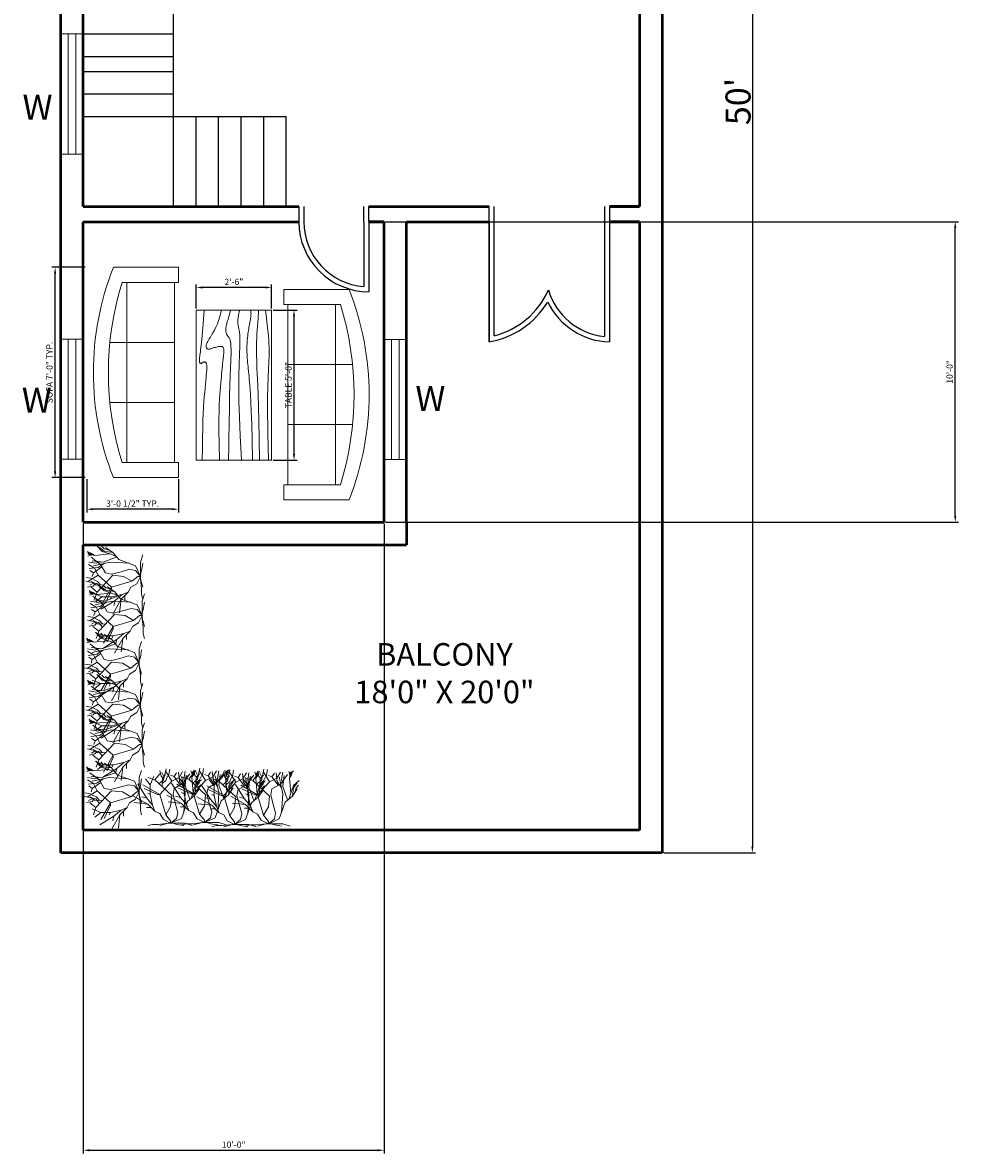
# Model space of a CAD drawing. Units: inches. Extents: x 995 to 2141, y 2161 to 2928.
# Tile 6 of 7: x 1768 to 2141, y 2161 to 2613. Entities that reach past the tile are written whole.
import ezdxf

# ---------------------------------------------------------------- set-up
doc = ezdxf.new("R2010")
doc.units = ezdxf.units.IN
for name, color, linetype, lineweight in [('A-ANNO-DIMS', 2, 'Continuous', 18), ('A-ANNO-TEXT', 7, 'Continuous', 18), ('A-AREA-IDEN', 7, 'Continuous', 25), ('A-DOOR', 3, 'Continuous', 25), ('A-FLOR-STRS', 7, 'Continuous', 25), ('A-FURN', 8, 'Continuous', 18), ('A-GLAZ', 4, 'Continuous', 18), ('A-WALL', 7, 'Continuous', 50), ('L-PLNT-TREE', 94, 'Continuous', 13)]:
    doc.layers.add(name, color=color, linetype=linetype, lineweight=lineweight)
doc.styles.get("Standard").update_dxf_attribs({"font": 'arial.ttf'})
doc.dimstyles.new('ISO-25', dxfattribs={"dimtxt": 2.5, "dimasz": 2.5, "dimexe": 1.25, "dimexo": 0.625, "dimtad": 1, "dimdec": 0, "dimlunit": 3, "dimtxsty": 'Standard', "dimcen": 2.5, "dimadec": 0, "dimazin": 0, "dimtfac": 1, "dimtdec": 0, "dimtmove": 0, "dimatfit": 3, "dimfxl": 1, "dimarcsym": 0})

# ---------------------------------------------------------------- blocks, each defined once
blk = doc.blocks.new('*U15')
for p, q in [((-11.433, 18.289), (-10.457, 22.749)), ((-9.48, 19.775), (-8.992, 22.592)), ((-16.8, 16.32), (-18.72, 18.72)), ((-14.88, 18.24), (-17.76, 19.2)), ((-16.8, 16.32), (-15.36, 19.68)), ((-14.88, 18.24), (-12.96, 20.64)), ((-8.16, 12), (-14.88, 18.24)), ((-13.325, 16.724), (-11.433, 18.289)), ((-12.471, 19.775), (-12.898, 22.044)), ((-11.677, 19.071), (-12.471, 19.775)), ((-11.28, 19.619), (-12.104, 21.184)), ((-12.043, 15.628), (-11.921, 18.836)), ((-11.921, 18.836), (-10.64, 20.401)), ((-10.579, 18.054), (-9.846, 19.697)), ((-8.16, 17.76), (-10.56, 21.6)), ((-7.2, 19.68), (-8.64, 20.16)), ((-8.16, 17.76), (-5.28, 19.2)), ((-7.2, 19.68), (-6.24, 21.12)), ((-4.8, 16.32), (-7.2, 19.68)), ((-5.086, 17.741), (-5.513, 21.34)), ((-5.28, 19.2), (-3.84, 21.6)), ((-2.88, 12.96), (-4.32, 19.68)), ((-3.84, 16.8), (-0.96, 20.64)), ((-3.377, 18.602), (-2.888, 21.575)), ((-2.766, 16.802), (-3.377, 18.602)), ((-2.88, 15.84), (-2.4, 20.16)), ((-0.508, 21.888), (-0.081, 20.558)), ((-0.203, 19.149), (0.102, 21.34)), ((0.346, 13.203), (-0.203, 19.149)), ((-0.142, 19.384), (0.59, 20.401)), ((-0.02, 20.01), (0.896, 21.105)), ((0.041, 20.714), (1.384, 22.044)), ((0.102, 21.34), (0.835, 21.888)), ((1.323, 16.254), (3.642, 18.289)), ((-18.24, 11.04), (-21.755, 16.655)), ((-12.96, 12.48), (-19.68, 16.32)), ((-13.92, 12.48), (-19.2, 14.88)), ((-16.8, 12.48), (-16.8, 16.32)), ((-12.96, 12.48), (-8.16, 17.76)), ((-11.982, 16.802), (-10.579, 18.054)), ((-7.68, 12.48), (-7.2, 14.88)), ((-7.2, 14.88), (-3.84, 16.8)), ((-3.377, 15.315), (-5.086, 17.819)), ((-0.96, 10.56), (-2.88, 15.84)), ((0.346, 13.203), (1.323, 16.254)), ((0.96, 12), (1.44, 15.36)), ((0.96, 12), (2.88, 14.88)), ((1.44, 15.36), (2.88, 17.28)), ((1.92, 13.44), (2.4, 15.36)), ((2.4, 15.36), (3.36, 16.32)), ((-17.76, 8.64), (-23.663, 11.961)), ((-17.76, 8.64), (-23.128, 9.222)), ((-18.24, 11.04), (-20.16, 11.52)), ((-15.84, 8.16), (-18.24, 11.04)), ((-16.8, 12.48), (-17.76, 12.96)), ((-15.84, 8.16), (-16.8, 12.48)), ((-12.96, 12.48), (-13.92, 12.48)), ((-10.56, 4.32), (-12.96, 12.48)), ((-8.64, 7.68), (-8.16, 12)), ((-6.72, 8.64), (-7.68, 12.48)), ((-4.32, 2.88), (-1.92, 9.6)), ((-3.36, 5.28), (-2.88, 12.96)), ((-1.92, 9.6), (0.96, 12)), ((-0.48, 10.8), (0.346, 13.203)), ((-16.32, 7.2), (-18.24, 7.2)), ((-14.88, 5.76), (-17.76, 8.64)), ((-14.88, 5.76), (-15.84, 8.16)), ((-12.96, 4.8), (-14.88, 5.76)), ((-11.52, 2.4), (-12.96, 4.8)), ((-10.56, 4.32), (-8.64, 7.68)), ((-5.76, 5.28), (-6.72, 8.64)), ((-6.24, 2.88), (-5.76, 5.28)), ((-15.84, 0.48), (-17.76, 0)), ((-13.44, 0.48), (-15.84, 0.48)), ((-9.6, 0.96), (-13.44, 0.48)), ((-9.6, 0.96), (-12.96, 0)), ((-8.64, 0.96), (-11.52, 2.4)), ((-8.64, 1.92), (-10.56, 4.32)), ((-9.6, 0.96), (-7.68, 0.96)), ((-8.64, 0.96), (-4.32, 2.88)), ((-8.64, 0.96), (-6.24, 2.88)), ((-8.64, 0.96), (-8.64, 1.92)), ((-8.64, 0.96), (-2.88, 0.96)), ((-7.68, 0.96), (-6.24, 0.48)), ((-6.24, 0.48), (-3.36, 0)), ((-2.88, 0.96), (0, 0))]:
    blk.add_line(p, q)
blk = doc.blocks.new('Sofa - Roundback 7 ft.')
for p, q in [((-12.00002, -32.4421), (-12.00003, -6.5971)), ((11.99997, -32.4421), (11.99998, -6.5971)), ((-36.000027, -34), (-36.000027, -11.4696)), ((-35.999844, -13.3819), (35.9998, -13.3819)), ((35.99998, -34), (35.99998, -11.4696)), ((-36.000027, -32.4421), (35.99998, -32.4421))]:
    blk.add_line(p, q)
for points in [[(-36.000027, -34), (-42.000027, -34), (-42.000027, -8)], [(41.99998, -8), (41.99998, -34), (35.99998, -34)]]:
    blk.add_lwpolyline(points)
for centre, radius, start, end in [((0, -114.25), 114.25, 68.43141, 111.5686), ((-0.00001, -127.1968), 121.1968, 72.72033, 107.2797)]:
    blk.add_arc(centre, radius, start, end)
blk = doc.blocks.new('Table - Rectangular Woodgrain 60 x 30 in.')
for p, q in [((0, 0), (0, -30)), ((60, 0), (0, 0)), ((60, -30), (60, 0)), ((0, -30), (60, -30))]:
    blk.add_line(p, q)
for points in [[(0, -2.4), (4.8155, -2.418), (9.0302, -2.4688), (12.709, -2.5477), (15.9167, -2.65), (18.7181, -2.7711), (21.1781, -2.9063), (23.3616, -3.0508), (25.3333, -3.2), (27.1477, -3.3495), (28.8172, -3.4958), (30.3437, -3.636), (31.7291, -3.7667), (32.9756, -3.8849), (34.0849, -3.9875), (35.059, -4.0714), (35.9, -4.1334), (36.6114, -4.1711), (37.2041, -4.1854), (37.6906, -4.1779), (38.0833, -4.15), (38.3948, -4.1034), (38.6375, -4.0396), (38.8239, -3.9602), (38.9666, -3.8667), (39.0764, -3.7608), (39.1573, -3.6448), (39.2116, -3.521), (39.2416, -3.3917), (39.2498, -3.2593), (39.2385, -3.1261), (39.21, -2.9944), (39.1666, -2.8667), (39.111, -2.7447), (39.0468, -2.6281), (38.978, -2.5163), (38.9083, -2.4083), (38.8418, -2.3035), (38.7823, -2.201), (38.7337, -2.1001), (38.7, -2), (38.6844, -1.9003), (38.6875, -1.8021), (38.7094, -1.707), (38.75, -1.6167), (38.8094, -1.5326), (38.8875, -1.4563), (38.9844, -1.3893), (39.1, -1.3333), (39.2351, -1.2896), (39.3937, -1.2583), (39.5804, -1.2396), (39.8, -1.2333), (40.057, -1.2396), (40.3562, -1.2583), (40.7023, -1.2896), (41.1, -1.3333), (41.5547, -1.3895), (42.0755, -1.4573), (42.6721, -1.5361), (43.3542, -1.625), (44.1316, -1.7233), (45.014, -1.8302), (46.0114, -1.9449), (47.1333, -2.0667), (48.3862, -2.1947), (49.7625, -2.3281), (51.2513, -2.4663), (52.8416, -2.6083), (54.5226, -2.7535), (56.2833, -2.9011), (58.1127, -3.0501), (60, -3.2)], [(0, -9.2), (6.5759, -9.0858), (11.9385, -9.0365), (16.2527, -9.0418), (19.6833, -9.0917), (22.3952, -9.1759), (24.5531, -9.2844), (26.322, -9.4069), (27.8666, -9.5333), (29.3241, -9.6553), (30.7203, -9.7719), (32.0532, -9.8837), (33.3208, -9.9917), (34.5213, -10.0965), (35.6526, -10.199), (36.7128, -10.2999), (37.7, -10.4), (38.6129, -10.4996), (39.4531, -10.5969), (40.223, -10.6895), (40.925, -10.775), (41.5613, -10.8512), (42.1344, -10.9156), (42.6465, -10.966), (43.1, -11), (43.4976, -11.0158), (43.8437, -11.0136), (44.143, -10.9942), (44.4, -10.9583), (44.6195, -10.9069), (44.8062, -10.8406), (44.9648, -10.7603), (45.1, -10.6667), (45.2155, -10.5598), (45.3114, -10.4365), (45.3871, -10.2929), (45.4416, -10.125), (45.4743, -9.929), (45.4844, -9.7011), (45.4709, -9.4371), (45.4333, -9.1333), (45.3716, -8.7883), (45.2896, -8.4104), (45.1919, -8.0107), (45.0833, -7.6), (44.9685, -7.1893), (44.8521, -6.7896), (44.7388, -6.4117), (44.6333, -6.0667), (44.54, -5.7628), (44.4614, -5.4979), (44.4001, -5.2675), (44.3583, -5.0667), (44.3384, -4.8909), (44.3427, -4.7354), (44.3736, -4.5956), (44.4333, -4.4667), (44.5236, -4.3453), (44.6427, -4.2333), (44.7884, -4.1339), (44.9583, -4.05), (45.1501, -3.9849), (45.3614, -3.9417), (45.59, -3.9234), (45.8333, -3.9333), (46.0915, -3.9749), (46.3734, -4.0531), (46.6906, -4.1736), (47.0542, -4.3417), (47.4756, -4.5629), (47.9661, -4.8427), (48.5372, -5.1866), (49.2, -5.6), (49.9676, -6.0844), (50.8594, -6.625), (51.8965, -7.2031), (53.1, -7.8), (54.491, -8.3969), (56.0906, -8.975), (57.9199, -9.5156), (60, -10)], [(0, -12.8), (5.1847, -12.9322), (9.6213, -13.0323), (13.3963, -13.1059), (16.5958, -13.1583), (19.3063, -13.1952), (21.614, -13.2219), (23.6054, -13.2439), (25.3666, -13.2667), (26.9728, -13.2947), (28.4531, -13.3281), (29.8256, -13.3663), (31.1083, -13.4083), (32.3191, -13.4535), (33.476, -13.501), (34.597, -13.5501), (35.7, -13.6), (36.7984, -13.6497), (37.8875, -13.6979), (38.9578, -13.743), (40, -13.7833), (41.0047, -13.8174), (41.9625, -13.8438), (42.864, -13.8607), (43.7, -13.8667), (44.4631, -13.8604), (45.1552, -13.8417), (45.7801, -13.8104), (46.3416, -13.7667), (46.8439, -13.7104), (47.2906, -13.6417), (47.6858, -13.5604), (48.0333, -13.4667), (48.3375, -13.3608), (48.6042, -13.2448), (48.8396, -13.121), (49.05, -12.9917), (49.2417, -12.8593), (49.4208, -12.7261), (49.5937, -12.5944), (49.7667, -12.4667), (49.9452, -12.3451), (50.1323, -12.2313), (50.3303, -12.1268), (50.5416, -12.0333), (50.7686, -11.9524), (51.0135, -11.8854), (51.2788, -11.8341), (51.5666, -11.8), (51.8785, -11.7843), (52.2116, -11.7865), (52.562, -11.8059), (52.926, -11.8417), (53.2998, -11.8931), (53.6795, -11.9594), (54.0614, -12.0397), (54.4416, -12.1333), (54.8223, -12.2401), (55.2293, -12.3625), (55.6942, -12.5037), (56.2489, -12.6667), (56.9251, -12.8547), (57.7545, -13.0708), (58.7689, -13.3182), (60, -13.6)], [(0, -18), (5.124, -17.7273), (9.6609, -17.5057), (13.6705, -17.3303), (17.2125, -17.1958), (20.3467, -17.0973), (23.1328, -17.0297), (25.6307, -16.9878), (27.9, -16.9667), (29.9928, -16.9617), (31.9302, -16.9703), (33.7254, -16.9907), (35.3917, -17.0208), (36.9423, -17.0588), (38.3906, -17.1026), (39.7499, -17.1503), (41.0333, -17.2), (42.2519, -17.2496), (43.4073, -17.2969), (44.4986, -17.3395), (45.525, -17.375), (46.4858, -17.4012), (47.3802, -17.4156), (48.2074, -17.416), (48.9667, -17.4), (49.6583, -17.3662), (50.2872, -17.3167), (50.8595, -17.2547), (51.3812, -17.1833), (51.8584, -17.1057), (52.2971, -17.025), (52.7034, -16.9443), (53.0833, -16.8667), (53.443, -16.7951), (53.789, -16.7313), (54.128, -16.6768), (54.4666, -16.6334), (54.8115, -16.6024), (55.1693, -16.5854), (55.5465, -16.5841), (55.95, -16.6), (56.3828, -16.6337), (56.8346, -16.6823), (57.2915, -16.7418), (57.7396, -16.8084), (58.165, -16.878), (58.5539, -16.9469), (58.8924, -17.0111), (59.1666, -17.0667), (59.3679, -17.1107), (59.5078, -17.1438), (59.6032, -17.1675), (59.6708, -17.1833), (59.7275, -17.193), (59.7901, -17.1979), (59.8753, -17.1998), (60, -17.2)], [(0, -22.4), (8.0098, -22.2501), (14.4094, -22.1011), (19.4168, -21.9535), (23.25, -21.8083), (26.1269, -21.6663), (28.2656, -21.5281), (29.884, -21.3947), (31.2, -21.2667), (32.3967, -21.1448), (33.5172, -21.0292), (34.5697, -20.9198), (35.5625, -20.8167), (36.5037, -20.7198), (37.4015, -20.6292), (38.2642, -20.5448), (39.1, -20.4667), (39.9164, -20.3951), (40.7187, -20.3313), (41.5117, -20.2768), (42.3, -20.2333), (43.0883, -20.2024), (43.8812, -20.1854), (44.6836, -20.1841), (45.5, -20.2), (46.3328, -20.234), (47.1747, -20.2844), (48.0163, -20.3488), (48.8479, -20.425), (49.66, -20.5106), (50.4429, -20.6031), (51.1872, -20.7004), (51.8833, -20.8), (52.5246, -20.8999), (53.1166, -20.9995), (53.6681, -21.0983), (54.1875, -21.1958), (54.6834, -21.2919), (55.1646, -21.3859), (55.6394, -21.4777), (56.1167, -21.5667), (56.6028, -21.6515), (57.0961, -21.7266), (57.5929, -21.7852), (58.0896, -21.8208), (58.5823, -21.8268), (59.0674, -21.7964), (59.5412, -21.723), (60, -21.6)], [(0, -25.2), (8.6355, -25.0504), (15.7026, -24.9031), (21.4049, -24.7606), (25.9458, -24.625), (29.529, -24.4988), (32.3578, -24.3844), (34.6359, -24.284), (36.5667, -24.2), (38.3213, -24.1341), (39.9417, -24.0854), (41.437, -24.0523), (42.8167, -24.0333), (44.0901, -24.0268), (45.2667, -24.0313), (46.3557, -24.0451), (47.3667, -24.0667), (48.309, -24.0947), (49.1928, -24.1287), (50.0284, -24.168), (50.826, -24.2125), (51.5959, -24.2617), (52.3483, -24.3151), (53.0935, -24.3725), (53.8417, -24.4334), (54.6009, -24.497), (55.3699, -24.561), (56.1454, -24.6226), (56.9239, -24.6792), (57.7021, -24.7279), (58.4764, -24.7662), (59.2435, -24.7911), (60, -24.8)], [(0, -28.8), (5.6867, -28.6681), (10.45, -28.5698), (14.407, -28.5012), (17.675, -28.4584), (20.3711, -28.4374), (22.6125, -28.4344), (24.5164, -28.4455), (26.2, -28.4667), (27.762, -28.4947), (29.2276, -28.5281), (30.6033, -28.5663), (31.8958, -28.6084), (33.1118, -28.6535), (34.2578, -28.7011), (35.3405, -28.7501), (36.3666, -28.8), (37.3443, -28.8497), (38.288, -28.8974), (39.2137, -28.9412), (40.1375, -28.9792), (41.0753, -29.0093), (42.0432, -29.0297), (43.0572, -29.0384), (44.1333, -29.0333), (45.2936, -29.0114), (46.5843, -28.9641), (48.0579, -28.8816), (49.7666, -28.7542), (51.7629, -28.5721), (54.0989, -28.3255), (56.8272, -28.0048), (60, -27.6)]]:
    blk.add_lwpolyline(points)
blk = doc.blocks.new('*D20')
at = {"layer": 'A-ANNO-DIMS', "color": 0, "lineweight": -2, "transparency": 16777216}
for p, q in [((2023.72, 2881.1), (2060.35, 2881.1)), ((2059.1, 2878.6), (2059.1, 2283.6)), ((2023.72, 2281.1), (2060.35, 2281.1))]:
    blk.add_line(p, q, dxfattribs=at)
at = {"layer": 'A-ANNO-DIMS', "color": 0, "transparency": 16777216}
for points in [[(2058.68, 2878.6), (2059.51, 2878.6), (2059.1, 2881.1)], [(2058.68, 2283.6), (2059.51, 2283.6), (2059.1, 2281.1)]]:
    blk.add_solid(points, dxfattribs=at)
at = {"layer": 'Defpoints', "color": 0, "transparency": 16777216}
for p in [(2023.1, 2881.1), (2023.1, 2281.1), (2059.1, 2281.1)]:
    blk.add_point(p, dxfattribs=at)
at = {"layer": 'A-ANNO-DIMS', "color": 0, "transparency": 16777216, "insert": (2053.37, 2581.1), "char_height": 2.5, "attachment_point": 5, "rotation": 90}
blk.add_mtext("{\\H4x;50'}", dxfattribs=at)
blk = doc.blocks.new('WIN-48IN')
for p, q in [((0, 48), (0, 0)), ((9, 48), (0, 48)), ((3, 48), (3, 0)), ((6, 0), (6, 48)), ((9, 0), (9, 48)), ((0, 0), (9, 0))]:
    blk.add_line(p, q)
blk = doc.blocks.new('*D48')
at = {"layer": 'A-ANNO-DIMS', "color": 0, "lineweight": -2, "transparency": 16777216}
for p, q in [((1792.82, 2514.88), (1779.59, 2514.88)), ((1780.84, 2433.38), (1780.84, 2512.38)), ((1792.82, 2430.88), (1779.59, 2430.88))]:
    blk.add_line(p, q, dxfattribs=at)
at = {"layer": 'A-ANNO-DIMS', "color": 0, "transparency": 16777216}
for points in [[(1780.42, 2512.38), (1781.26, 2512.38), (1780.84, 2514.88)], [(1780.42, 2433.38), (1781.26, 2433.38), (1780.84, 2430.88)]]:
    blk.add_solid(points, dxfattribs=at)
at = {"layer": 'Defpoints', "color": 0, "transparency": 16777216}
for p in [(1780.84, 2514.88), (1793.44, 2514.88), (1793.44, 2430.88)]:
    blk.add_point(p, dxfattribs=at)
at = {"layer": 'A-ANNO-DIMS', "color": 0, "transparency": 16777216, "insert": (1778.92, 2472.88), "char_height": 2.5, "attachment_point": 5, "rotation": 90}
blk.add_mtext('SOFA 7\'-0" TYP.', dxfattribs=at)
blk = doc.blocks.new('*D49')
at = {"layer": 'A-ANNO-DIMS', "color": 0, "lineweight": -2, "transparency": 16777216}
for p, q in [((1793.44, 2430.26), (1793.44, 2417.03)), ((1830.11, 2430.26), (1830.11, 2417.03)), ((1827.61, 2418.28), (1795.94, 2418.28))]:
    blk.add_line(p, q, dxfattribs=at)
at = {"layer": 'A-ANNO-DIMS', "color": 0, "transparency": 16777216}
for points in [[(1795.94, 2418.7), (1795.94, 2417.87), (1793.44, 2418.28)], [(1827.61, 2418.7), (1827.61, 2417.87), (1830.11, 2418.28)]]:
    blk.add_solid(points, dxfattribs=at)
at = {"layer": 'Defpoints', "color": 0, "transparency": 16777216}
for p in [(1793.44, 2430.88), (1830.11, 2430.88), (1793.44, 2418.28)]:
    blk.add_point(p, dxfattribs=at)
at = {"layer": 'A-ANNO-DIMS', "color": 0, "transparency": 16777216, "insert": (1811.77, 2420.2), "char_height": 2.5, "attachment_point": 5}
blk.add_mtext('3\'-0 1/2" TYP.', dxfattribs=at)
blk = doc.blocks.new('*D58')
at = {"layer": 'A-ANNO-DIMS', "color": 0, "lineweight": -2, "transparency": 16777216}
for p, q in [((1867.82, 2497.83), (1877.44, 2497.83)), ((1876.19, 2440.33), (1876.19, 2495.33)), ((1867.82, 2437.83), (1877.44, 2437.83))]:
    blk.add_line(p, q, dxfattribs=at)
at = {"layer": 'A-ANNO-DIMS', "color": 0, "transparency": 16777216}
for points in [[(1875.78, 2495.33), (1876.61, 2495.33), (1876.19, 2497.83)], [(1875.78, 2440.33), (1876.61, 2440.33), (1876.19, 2437.83)]]:
    blk.add_solid(points, dxfattribs=at)
at = {"layer": 'Defpoints', "color": 0, "transparency": 16777216}
for p in [(1867.19, 2497.83), (1876.19, 2497.83), (1867.19, 2437.83)]:
    blk.add_point(p, dxfattribs=at)
at = {"layer": 'A-ANNO-DIMS', "color": 0, "transparency": 16777216, "insert": (1874.29, 2467.83), "char_height": 2.5, "attachment_point": 5, "rotation": 90}
blk.add_mtext('TABLE 5\'-0"', dxfattribs=at)
blk = doc.blocks.new('*D59')
at = {"layer": 'A-ANNO-DIMS', "color": 0, "lineweight": -2, "transparency": 16777216}
for p, q in [((1837.19, 2498.45), (1837.19, 2508.08)), ((1864.69, 2506.83), (1839.69, 2506.83)), ((1867.19, 2498.45), (1867.19, 2508.08))]:
    blk.add_line(p, q, dxfattribs=at)
at = {"layer": 'A-ANNO-DIMS', "color": 0, "transparency": 16777216}
for points in [[(1839.69, 2507.24), (1839.69, 2506.41), (1837.19, 2506.83)], [(1864.69, 2507.24), (1864.69, 2506.41), (1867.19, 2506.83)]]:
    blk.add_solid(points, dxfattribs=at)
at = {"layer": 'Defpoints', "color": 0, "transparency": 16777216}
for p in [(1837.19, 2506.83), (1837.19, 2497.83), (1867.19, 2497.83)]:
    blk.add_point(p, dxfattribs=at)
at = {"layer": 'A-ANNO-DIMS', "color": 0, "transparency": 16777216, "insert": (1852.19, 2508.73), "char_height": 2.5, "attachment_point": 5}
blk.add_mtext('2\'-6"', dxfattribs=at)
blk = doc.blocks.new('*D62')
at = {"layer": 'A-ANNO-DIMS', "color": 0, "lineweight": -2, "transparency": 16777216}
for p, q in [((1792.1, 2412.48), (1792.1, 2161.03)), ((1912.1, 2412.48), (1912.1, 2161.03)), ((1794.6, 2162.28), (1909.6, 2162.28))]:
    blk.add_line(p, q, dxfattribs=at)
at = {"layer": 'A-ANNO-DIMS', "color": 0, "transparency": 16777216}
for points in [[(1794.6, 2162.69), (1794.6, 2161.86), (1792.1, 2162.28)], [(1909.6, 2162.69), (1909.6, 2161.86), (1912.1, 2162.28)]]:
    blk.add_solid(points, dxfattribs=at)
at = {"layer": 'Defpoints', "color": 0, "transparency": 16777216}
for p in [(1792.1, 2413.1), (1912.1, 2413.1), (1912.1, 2162.28)]:
    blk.add_point(p, dxfattribs=at)
at = {"layer": 'A-ANNO-DIMS', "color": 0, "transparency": 16777216, "insert": (1852.1, 2164.18), "char_height": 2.5, "attachment_point": 5}
blk.add_mtext('10\'-0"', dxfattribs=at)
blk = doc.blocks.new('*D63')
at = {"layer": 'A-ANNO-DIMS', "color": 0, "lineweight": -2, "transparency": 16777216}
for p, q in [((1912.72, 2533.1), (2141.3, 2533.1)), ((2140.05, 2415.6), (2140.05, 2530.6)), ((1912.72, 2413.1), (2141.3, 2413.1))]:
    blk.add_line(p, q, dxfattribs=at)
at = {"layer": 'A-ANNO-DIMS', "color": 0, "transparency": 16777216}
for points in [[(2139.63, 2530.6), (2140.46, 2530.6), (2140.05, 2533.1)], [(2139.63, 2415.6), (2140.46, 2415.6), (2140.05, 2413.1)]]:
    blk.add_solid(points, dxfattribs=at)
at = {"layer": 'Defpoints', "color": 0, "transparency": 16777216}
for p in [(1912.1, 2533.1), (2140.05, 2533.1), (1912.1, 2413.1)]:
    blk.add_point(p, dxfattribs=at)
at = {"layer": 'A-ANNO-DIMS', "color": 0, "transparency": 16777216, "insert": (2138.14, 2473.1), "char_height": 2.5, "attachment_point": 5, "rotation": 90}
blk.add_mtext('10\'-0"', dxfattribs=at)

msp = doc.modelspace()

# ---------------------------------------------------------------- linework, layer by layer
at = {"layer": 'A-DOOR'}
for p, q in [((1878.1, 2539.1), (1878.1, 2533.1)), ((1880.1, 2539.1), (1880.1, 2533.1)), ((1904.1, 2533.1), (1904.1, 2539.1)), ((1906.1, 2533.1), (1906.1, 2539.1)), ((1954.1, 2533.1), (1954.1, 2539.1)), ((1956.1, 2533.1), (1956.1, 2539.1)), ((2000.1, 2539.1), (2000.1, 2533.1)), ((2002.1, 2539.1), (2002.1, 2533.1)), ((2002.1, 2539.1), (2002.1, 2533.1)), ((1904.1, 2533.1), (1904.1, 2507.18)), ((1906.1, 2533.1), (1906.1, 2505.1)), ((1954.1, 2533.1), (1954.1, 2485.1)), ((1954.1, 2485.1), (1954.1, 2533.1)), ((1956.1, 2487.57), (1956.1, 2533.1)), ((2000.1, 2533.1), (2000.1, 2487.23)), ((2002.1, 2533.1), (2002.1, 2485.1))]:
    msp.add_line(p, q, dxfattribs=at)
for centre, radius, start, end in [((1906.1, 2533.1), 28, 180, 270), ((1906.1, 2533.1), 26, 180, 265.5883), ((1948.23, 2518.74), 32.15, 284.1675, 336.3358), ((2002.81, 2513.31), 26.22, 196.5614, 264.0668), ((1948.19, 2518.83), 34.24, 279.9424, 328.65), ((2002.77, 2513.23), 28.14, 205.7327, 268.6217)]:
    msp.add_arc(centre, radius, start, end, dxfattribs=at)
at = {"layer": 'A-FLOR-STRS'}
for p, q in [((1828.1, 2539.1), (1828.1, 2707.1)), ((1792.1, 2608.1), (1828.1, 2608.1)), ((1792.1, 2599.1), (1828.1, 2599.1)), ((1792.1, 2593.1), (1828.1, 2593.1)), ((1792.1, 2584.1), (1828.1, 2584.1)), ((1792.1, 2575.1), (1873.1, 2575.1)), ((1837.1, 2539.1), (1837.1, 2575.1)), ((1846.1, 2539.1), (1846.1, 2575.1)), ((1855.1, 2539.1), (1855.1, 2575.1)), ((1864.1, 2539.1), (1864.1, 2575.1)), ((1873.1, 2539.1), (1873.1, 2575.1))]:
    msp.add_line(p, q, dxfattribs=at)
at = {"layer": 'A-WALL'}
for p, q in [((1783.1, 2281.1), (1783.1, 2881.1)), ((2023.1, 2881.1), (2023.1, 2281.1)), ((1792.1, 2539.1), (1792.1, 2707.1)), ((2014.1, 2707.1), (2014.1, 2539.1)), ((1792.1, 2539.1), (1878.1, 2539.1)), ((1906.1, 2539.1), (1954.1, 2539.1)), ((2014.1, 2539.1), (2002.1, 2539.1)), ((2002.1, 2539.1), (2014.1, 2539.1)), ((1792.1, 2533.1), (1878.1, 2533.1)), ((1792.1, 2413.1), (1792.1, 2533.1)), ((1912.1, 2533.1), (1906.1, 2533.1)), ((1906.1, 2533.1), (1912.1, 2533.1)), ((1912.1, 2413.1), (1912.1, 2533.1)), ((1921.1, 2533.1), (1954.1, 2533.1)), ((1921.1, 2413.1), (1921.1, 2533.1)), ((2014.1, 2533.1), (2002.1, 2533.1)), ((2002.1, 2533.1), (2014.1, 2533.1)), ((2014.1, 2533.1), (2014.1, 2290.1)), ((1792.1, 2413.1), (1912.1, 2413.1)), ((1921.1, 2413.1), (1921.1, 2404.1)), ((1792.1, 2290.1), (1792.1, 2404.1)), ((1792.1, 2404.1), (1912.1, 2404.1)), ((1912.1, 2404.1), (1921.1, 2404.1)), ((2014.1, 2290.1), (1792.1, 2290.1)), ((2023.1, 2281.1), (1783.1, 2281.1))]:
    msp.add_line(p, q, dxfattribs=at)

# ---------------------------------------------------------------- block references
at = {"layer": 'A-FURN'}
for name, p, rotation in [('Sofa - Roundback 7 ft.', (1796.11, 2472.88), 90), ('Sofa - Roundback 7 ft.', (1906.14, 2464.05), 269.9999778309999), ('Table - Rectangular Woodgrain 60 x 30 in.', (1837.19, 2437.83), 90)]:
    msp.add_blockref(name, p, dxfattribs=dict(at, rotation=rotation))
at = {"layer": 'A-GLAZ'}
for p in [(1783.1, 2560.1), (1783.1, 2438.25), (1912.1, 2438.07)]:
    msp.add_blockref('WIN-48IN', p, dxfattribs=at)
at = {"layer": 'L-PLNT-TREE', "rotation": 90}
for p in [(1815.82, 2400.05), (1816.49, 2384.45), (1815.36, 2365.42), (1815.82, 2348.62), (1816.49, 2333.01), (1815.36, 2313.99)]:
    msp.add_blockref('*U15', p, dxfattribs=at)
at = {"layer": 'L-PLNT-TREE'}
for p in [(1835.57, 2291.91), (1849.08, 2292.17), (1861.08, 2291.45), (1874.59, 2291.71)]:
    msp.add_blockref('*U15', p, dxfattribs=at)

# ---------------------------------------------------------------- texts
at = {"layer": 'A-ANNO-TEXT', "char_height": 10, "attachment_point": 1}
for insert in [(1767.84, 2583.78), (1767.53, 2466.88), (1924.6, 2467.52)]:
    msp.add_mtext_dynamic_manual_height_columns('W', width=112.484, gutter_width=12.5, heights=[0], dxfattribs=dict(at, insert=insert))
at = {"layer": 'A-AREA-IDEN', "insert": (1877.07, 2364.8), "char_height": 9, "attachment_point": 1}
msp.add_mtext_dynamic_manual_height_columns('\\pxqc;BALCONY \\P18\'0" X 20\'0"', width=118.2971, gutter_width=12.5, heights=[0], dxfattribs=at)

# ---------------------------------------------------------------- dimensions: what is measured, and where the dimension line sits
at = {"layer": 'A-ANNO-DIMS'}
for base, p1, p2, angle, text, override, picture, middle in [((2059.1, 2281.1), (2023.1, 2881.1), (2023.1, 2281.1), 90, "{\\H4x;50'}", {"dimclrd": 0, "dimclre": 0, "dimclrt": 0}, '*D20', (2053.37, 2581.1)), ((1780.84, 2514.88), (1793.44, 2430.88), (1793.44, 2514.88), 90, 'SOFA <> TYP.', {"dimdec": 1, "dimlfac": 1, "dimrnd": 0, "dimzin": 1, "dimdsep": 46, "dimlunit": 4, "dimfrac": 2}, '*D48', (1778.92, 2472.88)), ((1876.19, 2497.83), (1867.19, 2437.83), (1867.19, 2497.83), 90, 'TABLE <>', {"dimdec": 1, "dimlfac": 1, "dimrnd": 0, "dimzin": 1, "dimdsep": 46, "dimlunit": 4, "dimfrac": 2}, '*D58', (1874.29, 2467.83)), ((1793.44, 2418.28), (1830.11, 2430.88), (1793.44, 2430.88), 180, '<> TYP.', {"dimdec": 1, "dimlfac": 1, "dimrnd": 0, "dimzin": 1, "dimdsep": 46, "dimlunit": 4, "dimfrac": 2}, '*D49', (1811.77, 2420.2))]:
    dim = msp.add_linear_dim(base=base, p1=p1, p2=p2, angle=angle, text=text, dimstyle='ISO-25', override=override, dxfattribs=at)
    dim.commit()
    dim.dimension.update_dxf_attribs({"geometry": picture, "text_midpoint": middle})
for base, p1, p2, angle, picture, middle in [((2140.05, 2533.1), (1912.1, 2413.1), (1912.1, 2533.1), 90, '*D63', (2138.14, 2473.1)), ((1837.19, 2506.83), (1867.19, 2497.83), (1837.19, 2497.83), 180, '*D59', (1852.19, 2508.73))]:
    dim = msp.add_linear_dim(base=base, p1=p1, p2=p2, angle=angle, dimstyle='ISO-25', override={"dimdec": 1, "dimlfac": 1, "dimrnd": 0, "dimzin": 1, "dimdsep": 46, "dimlunit": 4, "dimfrac": 2}, dxfattribs=at)
    dim.commit()
    dim.dimension.update_dxf_attribs({"geometry": picture, "text_midpoint": middle})
dim = msp.add_linear_dim(base=(1912.1, 2162.28), p1=(1792.1, 2413.1), p2=(1912.1, 2413.1), dimstyle='ISO-25', override={"dimdec": 1, "dimlfac": 1, "dimrnd": 0, "dimzin": 1, "dimdsep": 46, "dimlunit": 4, "dimfrac": 2}, dxfattribs=at)
dim.commit()
dim.dimension.update_dxf_attribs({"geometry": '*D62', "text_midpoint": (1852.1, 2164.18)})

doc.saveas('drawing.dxf')
